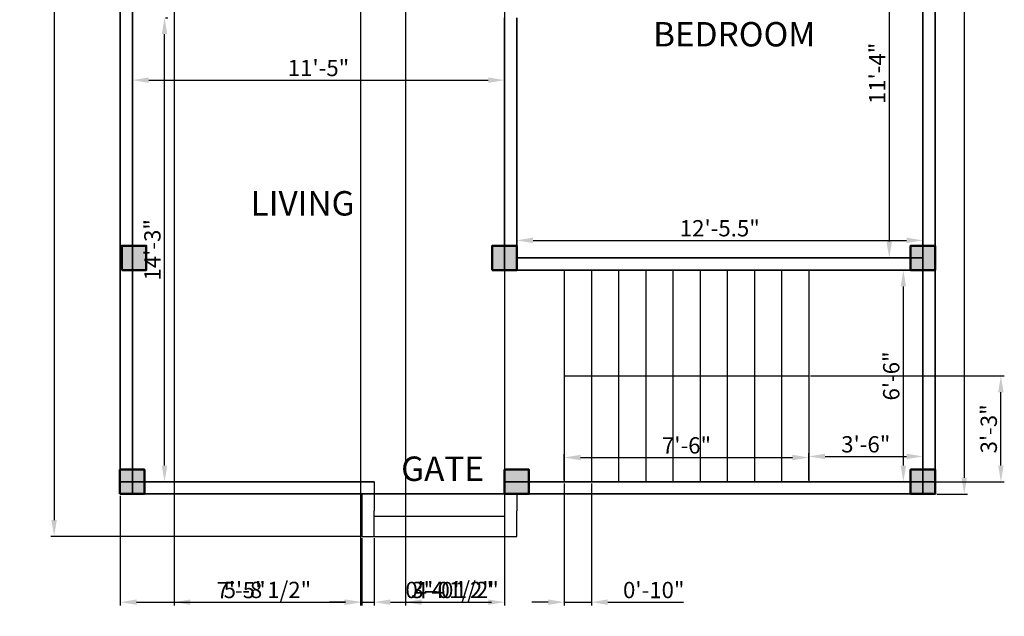
# Model space of a CAD drawing. Units: inches. Extents: x 6892 to 7255, y 6029 to 6556.
# Tile 1 of 2: x 6892 to 7255, y 6029 to 6249. Entities that reach past the tile are written whole.
import ezdxf

# ---------------------------------------------------------------- set-up
doc = ezdxf.new("R2010")
doc.units = ezdxf.units.IN
for name, color, linetype, lineweight in [('A-ANNO-DIMS', 2, 'Continuous', 18), ('A-ANNO-TEXT', 7, 'Continuous', 18), ('A-AREA-IDEN', 7, 'Continuous', 25), ('A-COLS', 7, 'Continuous', 50), ('A-COLS-PATT', 1, 'Continuous', 13), ('A-FLOR-STRS', 7, 'Continuous', 25), ('A-WALL', 7, 'Continuous', 35)]:
    doc.layers.add(name, color=color, linetype=linetype, lineweight=lineweight)
doc.styles.get("Standard").update_dxf_attribs({"font": 'arial.ttf'})
doc.dimstyles.new('ISO-25', dxfattribs={"dimtxt": 6, "dimasz": 6, "dimexe": 1.25, "dimexo": 0.625, "dimtad": 1, "dimlunit": 3, "dimtxsty": 'Standard', "dimcen": 2.5, "dimadec": 0, "dimazin": 0, "dimtfac": 1, "dimtmove": 0, "dimatfit": 3, "dimfxl": 1, "dimarcsym": 0})

# ---------------------------------------------------------------- blocks, each defined once
blk = doc.blocks.new('*D1')
at = {"layer": 'A-ANNO-DIMS', "color": 0, "lineweight": -2, "transparency": 16777216}
for p, q in [((6945.77, 6249.77), (6946.64, 6249.77)), ((6945.39, 6084.77), (6945.39, 6243.77)), ((6945.77, 6078.77), (6946.64, 6078.77))]:
    blk.add_line(p, q, dxfattribs=at)
at = {"layer": 'A-ANNO-DIMS', "color": 0, "transparency": 16777216}
for points in [[(6944.39, 6243.77), (6946.39, 6243.77), (6945.39, 6249.77)], [(6944.39, 6084.77), (6946.39, 6084.77), (6945.39, 6078.77)]]:
    blk.add_solid(points, dxfattribs=at)
at = {"layer": 'Defpoints', "color": 0, "transparency": 16777216}
for p in [(6945.15, 6249.77), (6945.39, 6249.77), (6945.15, 6078.77)]:
    blk.add_point(p, dxfattribs=at)
at = {"layer": 'A-ANNO-DIMS', "color": 0, "transparency": 16777216, "insert": (6941.7, 6164.27), "char_height": 6, "attachment_point": 5, "rotation": 90}
blk.add_mtext('14\'-3"', dxfattribs=at)
blk = doc.blocks.new('*D2')
at = {"layer": 'A-ANNO-DIMS', "color": 0, "lineweight": -2, "transparency": 16777216}
for p, q in [((6933.57, 6227.41), (6933.57, 6228.04)), ((6939.57, 6226.79), (7064.57, 6226.79)), ((7070.57, 6227.41), (7070.57, 6228.04))]:
    blk.add_line(p, q, dxfattribs=at)
at = {"layer": 'A-ANNO-DIMS', "color": 0, "transparency": 16777216}
for points in [[(6939.57, 6227.79), (6939.57, 6225.79), (6933.57, 6226.79)], [(7064.57, 6227.79), (7064.57, 6225.79), (7070.57, 6226.79)]]:
    blk.add_solid(points, dxfattribs=at)
at = {"layer": 'Defpoints', "color": 0, "transparency": 16777216}
for p in [(6933.57, 6226.79), (7070.57, 6226.79), (7070.57, 6226.79)]:
    blk.add_point(p, dxfattribs=at)
at = {"layer": 'A-ANNO-DIMS', "color": 0, "transparency": 16777216, "insert": (7002.07, 6230.48), "char_height": 6, "attachment_point": 5}
blk.add_mtext('11\'-5"', dxfattribs=at)
blk = doc.blocks.new('*D10')
at = {"layer": 'A-ANNO-DIMS', "color": 0, "lineweight": -2, "transparency": 16777216}
for p, q in [((7075.07, 6161.9), (7075.07, 6168.99)), ((7081.07, 6167.74), (7218.57, 6167.74)), ((7224.57, 6161.9), (7224.57, 6168.99))]:
    blk.add_line(p, q, dxfattribs=at)
at = {"layer": 'A-ANNO-DIMS', "color": 0, "transparency": 16777216}
for points in [[(7081.07, 6168.74), (7081.07, 6166.74), (7075.07, 6167.74)], [(7218.57, 6168.74), (7218.57, 6166.74), (7224.57, 6167.74)]]:
    blk.add_solid(points, dxfattribs=at)
at = {"layer": 'Defpoints', "color": 0, "transparency": 16777216}
for p in [(7224.57, 6167.74), (7075.07, 6161.27), (7224.57, 6161.27)]:
    blk.add_point(p, dxfattribs=at)
at = {"layer": 'A-ANNO-DIMS', "color": 0, "transparency": 16777216, "insert": (7149.82, 6171.43), "char_height": 6, "attachment_point": 5}
blk.add_mtext('12\'-5.5"', dxfattribs=at)
blk = doc.blocks.new('*D11')
at = {"layer": 'A-ANNO-DIMS', "color": 0, "lineweight": -2, "transparency": 16777216}
for p, q in [((7223.95, 6297.27), (7210.95, 6297.27)), ((7212.2, 6291.27), (7212.2, 6167.27)), ((7223.95, 6161.27), (7210.95, 6161.27))]:
    blk.add_line(p, q, dxfattribs=at)
at = {"layer": 'A-ANNO-DIMS', "color": 0, "transparency": 16777216}
for points in [[(7211.2, 6291.27), (7213.2, 6291.27), (7212.2, 6297.27)], [(7211.2, 6167.27), (7213.2, 6167.27), (7212.2, 6161.27)]]:
    blk.add_solid(points, dxfattribs=at)
at = {"layer": 'Defpoints', "color": 0, "transparency": 16777216}
for p in [(7224.57, 6297.27), (7212.2, 6161.27), (7224.57, 6161.27)]:
    blk.add_point(p, dxfattribs=at)
at = {"layer": 'A-ANNO-DIMS', "color": 0, "transparency": 16777216, "insert": (7208.56, 6229.27), "char_height": 6, "attachment_point": 5, "rotation": 90}
blk.add_mtext('11\'-4"', dxfattribs=at)
blk = doc.blocks.new('*D12')
at = {"layer": 'A-ANNO-DIMS', "color": 0, "lineweight": -2, "transparency": 16777216}
for p, q in [((7092.57, 6079.4), (7092.57, 6088.96)), ((7098.57, 6087.71), (7176.57, 6087.71)), ((7182.57, 6079.4), (7182.57, 6088.96))]:
    blk.add_line(p, q, dxfattribs=at)
at = {"layer": 'A-ANNO-DIMS', "color": 0, "transparency": 16777216}
for points in [[(7098.57, 6088.71), (7098.57, 6086.71), (7092.57, 6087.71)], [(7176.57, 6088.71), (7176.57, 6086.71), (7182.57, 6087.71)]]:
    blk.add_solid(points, dxfattribs=at)
at = {"layer": 'Defpoints', "color": 0, "transparency": 16777216}
for p in [(7182.57, 6087.71), (7092.57, 6078.77), (7182.57, 6078.77)]:
    blk.add_point(p, dxfattribs=at)
at = {"layer": 'A-ANNO-DIMS', "color": 0, "transparency": 16777216, "insert": (7137.57, 6091.4), "char_height": 6, "attachment_point": 5}
blk.add_mtext('7\'-6"', dxfattribs=at)
blk = doc.blocks.new('*D13')
at = {"layer": 'A-ANNO-DIMS', "color": 0, "lineweight": -2, "transparency": 16777216}
for p, q in [((7182.57, 6079.4), (7182.57, 6089.37)), ((7188.57, 6088.12), (7218.57, 6088.12)), ((7224.57, 6079.4), (7224.57, 6089.37))]:
    blk.add_line(p, q, dxfattribs=at)
at = {"layer": 'A-ANNO-DIMS', "color": 0, "transparency": 16777216}
for points in [[(7188.57, 6089.12), (7188.57, 6087.12), (7182.57, 6088.12)], [(7218.57, 6089.12), (7218.57, 6087.12), (7224.57, 6088.12)]]:
    blk.add_solid(points, dxfattribs=at)
at = {"layer": 'Defpoints', "color": 0, "transparency": 16777216}
for p in [(7224.57, 6088.12), (7182.57, 6078.77), (7224.57, 6078.77)]:
    blk.add_point(p, dxfattribs=at)
at = {"layer": 'A-ANNO-DIMS', "color": 0, "transparency": 16777216, "insert": (7203.57, 6091.81), "char_height": 6, "attachment_point": 5}
blk.add_mtext('3\'-6"', dxfattribs=at)
blk = doc.blocks.new('*D14')
at = {"layer": 'A-ANNO-DIMS', "color": 0, "lineweight": -2, "transparency": 16777216}
for p, q in [((7223.95, 6156.77), (7216.16, 6156.77)), ((7217.41, 6084.77), (7217.41, 6150.77)), ((7223.95, 6078.77), (7216.16, 6078.77))]:
    blk.add_line(p, q, dxfattribs=at)
at = {"layer": 'A-ANNO-DIMS', "color": 0, "transparency": 16777216}
for points in [[(7216.41, 6150.77), (7218.41, 6150.77), (7217.41, 6156.77)], [(7216.41, 6084.77), (7218.41, 6084.77), (7217.41, 6078.77)]]:
    blk.add_solid(points, dxfattribs=at)
at = {"layer": 'Defpoints', "color": 0, "transparency": 16777216}
for p in [(7217.41, 6156.77), (7224.57, 6156.77), (7224.57, 6078.77)]:
    blk.add_point(p, dxfattribs=at)
at = {"layer": 'A-ANNO-DIMS', "color": 0, "transparency": 16777216, "insert": (7213.72, 6117.77), "char_height": 6, "attachment_point": 5, "rotation": 90}
blk.add_mtext('6\'-6"', dxfattribs=at)
blk = doc.blocks.new('*D16')
at = {"layer": 'A-ANNO-DIMS', "color": 0, "lineweight": -2, "transparency": 16777216}
for p, q in [((7229.7, 6506.27), (7241.06, 6506.27)), ((7239.81, 6500.27), (7239.81, 6080.27)), ((7229.7, 6074.27), (7241.06, 6074.27))]:
    blk.add_line(p, q, dxfattribs=at)
at = {"layer": 'A-ANNO-DIMS', "color": 0, "transparency": 16777216}
for points in [[(7238.81, 6500.27), (7240.81, 6500.27), (7239.81, 6506.27)], [(7238.81, 6080.27), (7240.81, 6080.27), (7239.81, 6074.27)]]:
    blk.add_solid(points, dxfattribs=at)
at = {"layer": 'Defpoints', "color": 0, "transparency": 16777216}
for p in [(7229.07, 6506.27), (7229.07, 6074.27), (7239.81, 6074.27)]:
    blk.add_point(p, dxfattribs=at)
at = {"layer": 'A-ANNO-DIMS', "color": 0, "transparency": 16777216, "insert": (7236.12, 6290.27), "char_height": 6, "attachment_point": 5, "rotation": 90}
blk.add_mtext("36'", dxfattribs=at)
blk = doc.blocks.new('COL-9IN-SQ')
blk.add_lwpolyline([(0, 0), (9, 0), (9, 9), (0, 9)], close=True)
blk = doc.blocks.new('*D20')
at = {"layer": 'A-ANNO-DIMS', "color": 0, "lineweight": -2, "transparency": 16777216}
for p, q in [((6928.45, 6506.27), (6903.48, 6506.27)), ((6904.73, 6500.27), (6904.73, 6064.66)), ((7017.45, 6058.66), (6903.48, 6058.66))]:
    blk.add_line(p, q, dxfattribs=at)
at = {"layer": 'A-ANNO-DIMS', "color": 0, "transparency": 16777216}
for points in [[(6903.73, 6500.27), (6905.73, 6500.27), (6904.73, 6506.27)], [(6903.73, 6064.66), (6905.73, 6064.66), (6904.73, 6058.66)]]:
    blk.add_solid(points, dxfattribs=at)
at = {"layer": 'Defpoints', "color": 0, "transparency": 16777216}
for p in [(6929.07, 6506.27), (6904.73, 6058.66), (7018.07, 6058.66)]:
    blk.add_point(p, dxfattribs=at)
at = {"layer": 'A-ANNO-DIMS', "color": 0, "transparency": 16777216, "insert": (6901, 6282.47), "char_height": 6, "attachment_point": 5, "rotation": 90}
blk.add_mtext('37\'-3 1/2"', dxfattribs=at)
blk = doc.blocks.new('*D21')
at = {"layer": 'A-ANNO-DIMS', "color": 0, "lineweight": -2, "transparency": 16777216}
for p, q in [((7022.57, 6058.04), (7022.57, 6033.16)), ((7070.57, 6058.04), (7070.57, 6033.16)), ((7028.57, 6034.41), (7064.57, 6034.41))]:
    blk.add_line(p, q, dxfattribs=at)
at = {"layer": 'A-ANNO-DIMS', "color": 0, "transparency": 16777216}
for points in [[(7028.57, 6035.41), (7028.57, 6033.41), (7022.57, 6034.41)], [(7064.57, 6035.41), (7064.57, 6033.41), (7070.57, 6034.41)]]:
    blk.add_solid(points, dxfattribs=at)
at = {"layer": 'Defpoints', "color": 0, "transparency": 16777216}
for p in [(7022.57, 6058.66), (7070.57, 6058.66), (7070.57, 6034.41)]:
    blk.add_point(p, dxfattribs=at)
at = {"layer": 'A-ANNO-DIMS', "color": 0, "transparency": 16777216, "insert": (7046.57, 6038.1), "char_height": 6, "attachment_point": 5}
blk.add_mtext('4\'-0"', dxfattribs=at)
blk = doc.blocks.new('*D22')
at = {"layer": 'A-ANNO-DIMS', "color": 0, "lineweight": -2, "transparency": 16777216}
for p, q in [((7034.07, 6355.65), (7034.07, 6033.16)), ((7070.6, 6351.27), (7070.6, 6033.16)), ((7040.07, 6034.41), (7064.6, 6034.41))]:
    blk.add_line(p, q, dxfattribs=at)
at = {"layer": 'A-ANNO-DIMS', "color": 0, "transparency": 16777216}
for points in [[(7040.07, 6035.41), (7040.07, 6033.41), (7034.07, 6034.41)], [(7064.6, 6035.41), (7064.6, 6033.41), (7070.6, 6034.41)]]:
    blk.add_solid(points, dxfattribs=at)
at = {"layer": 'Defpoints', "color": 0, "transparency": 16777216}
for p in [(7034.07, 6356.27), (7070.6, 6351.9), (7070.6, 6034.41)]:
    blk.add_point(p, dxfattribs=at)
at = {"layer": 'A-ANNO-DIMS', "color": 0, "transparency": 16777216, "insert": (7052.34, 6038.14), "char_height": 6, "attachment_point": 5}
blk.add_mtext('3\'-0 1/2"', dxfattribs=at)
blk = doc.blocks.new('*D27')
at = {"layer": 'A-ANNO-DIMS', "color": 0, "lineweight": -2, "transparency": 16777216}
for p, q in [((7018.07, 6058.04), (7018.07, 6033.16)), ((7022.57, 6058.04), (7022.57, 6033.16)), ((7012.07, 6034.41), (7006.07, 6034.41)), ((7018.07, 6034.41), (7022.57, 6034.41)), ((7028.57, 6034.41), (7065.75, 6034.41))]:
    blk.add_line(p, q, dxfattribs=at)
at = {"layer": 'A-ANNO-DIMS', "color": 0, "transparency": 16777216}
for points in [[(7012.07, 6035.41), (7012.07, 6033.41), (7018.07, 6034.41)], [(7028.57, 6035.41), (7028.57, 6033.41), (7022.57, 6034.41)]]:
    blk.add_solid(points, dxfattribs=at)
at = {"layer": 'Defpoints', "color": 0, "transparency": 16777216}
for p in [(7018.07, 6058.66), (7022.57, 6058.66), (7022.57, 6034.41)]:
    blk.add_point(p, dxfattribs=at)
at = {"layer": 'A-ANNO-DIMS', "color": 0, "transparency": 16777216, "insert": (7050.16, 6038.14), "char_height": 6, "attachment_point": 5}
blk.add_mtext('0\'-4 1/2"', dxfattribs=at)
blk = doc.blocks.new('*D28')
at = {"layer": 'A-ANNO-DIMS', "color": 0, "lineweight": -2, "transparency": 16777216}
for p, q in [((6948.94, 6335.71), (6948.94, 6033.16)), ((7017.57, 6335.71), (7017.57, 6033.16)), ((6954.94, 6034.41), (7011.57, 6034.41))]:
    blk.add_line(p, q, dxfattribs=at)
at = {"layer": 'A-ANNO-DIMS', "color": 0, "transparency": 16777216}
for points in [[(6954.94, 6035.41), (6954.94, 6033.41), (6948.94, 6034.41)], [(7011.57, 6035.41), (7011.57, 6033.41), (7017.57, 6034.41)]]:
    blk.add_solid(points, dxfattribs=at)
at = {"layer": 'Defpoints', "color": 0, "transparency": 16777216}
for p in [(6948.94, 6336.33), (7017.57, 6336.33), (7017.57, 6034.41)]:
    blk.add_point(p, dxfattribs=at)
at = {"layer": 'A-ANNO-DIMS', "color": 0, "transparency": 16777216, "insert": (6983.26, 6038.14), "char_height": 6, "attachment_point": 5}
blk.add_mtext('5\'-8 1/2"', dxfattribs=at)
blk = doc.blocks.new('*D30')
at = {"layer": 'A-ANNO-DIMS', "color": 0, "lineweight": -2, "transparency": 16777216}
for p, q in [((7092.57, 6078.15), (7092.57, 6033.16)), ((7102.57, 6078.15), (7102.57, 6033.16)), ((7086.57, 6034.41), (7080.57, 6034.41)), ((7092.57, 6034.41), (7102.57, 6034.41)), ((7108.57, 6034.41), (7136.43, 6034.41))]:
    blk.add_line(p, q, dxfattribs=at)
at = {"layer": 'A-ANNO-DIMS', "color": 0, "transparency": 16777216}
for points in [[(7086.57, 6035.41), (7086.57, 6033.41), (7092.57, 6034.41)], [(7108.57, 6035.41), (7108.57, 6033.41), (7102.57, 6034.41)]]:
    blk.add_solid(points, dxfattribs=at)
at = {"layer": 'Defpoints', "color": 0, "transparency": 16777216}
for p in [(7092.57, 6078.77), (7102.57, 6078.77), (7102.57, 6034.41)]:
    blk.add_point(p, dxfattribs=at)
at = {"layer": 'A-ANNO-DIMS', "color": 0, "transparency": 16777216, "insert": (7125.5, 6038.1), "char_height": 6, "attachment_point": 5}
blk.add_mtext('0\'-10"', dxfattribs=at)
blk = doc.blocks.new('*D31')
at = {"layer": 'A-ANNO-DIMS', "color": 0, "lineweight": -2, "transparency": 16777216}
for p, q in [((7183.2, 6117.77), (7254.57, 6117.77)), ((7253.32, 6084.77), (7253.32, 6111.77)), ((7183.2, 6078.77), (7254.57, 6078.77))]:
    blk.add_line(p, q, dxfattribs=at)
at = {"layer": 'A-ANNO-DIMS', "color": 0, "transparency": 16777216}
for points in [[(7252.32, 6111.77), (7254.32, 6111.77), (7253.32, 6117.77)], [(7252.32, 6084.77), (7254.32, 6084.77), (7253.32, 6078.77)]]:
    blk.add_solid(points, dxfattribs=at)
at = {"layer": 'Defpoints', "color": 0, "transparency": 16777216}
for p in [(7182.57, 6117.77), (7253.32, 6117.77), (7182.57, 6078.77)]:
    blk.add_point(p, dxfattribs=at)
at = {"layer": 'A-ANNO-DIMS', "color": 0, "transparency": 16777216, "insert": (7249.63, 6098.27), "char_height": 6, "attachment_point": 5, "rotation": 90}
blk.add_mtext('3\'-3"', dxfattribs=at)
blk = doc.blocks.new('*D32')
at = {"layer": 'A-ANNO-DIMS', "color": 0, "lineweight": -2, "transparency": 16777216}
for p, q in [((6929.07, 6073.65), (6929.07, 6033.16)), ((7018.07, 6058.04), (7018.07, 6033.16)), ((6935.07, 6034.41), (7012.07, 6034.41))]:
    blk.add_line(p, q, dxfattribs=at)
at = {"layer": 'A-ANNO-DIMS', "color": 0, "transparency": 16777216}
for points in [[(6935.07, 6035.41), (6935.07, 6033.41), (6929.07, 6034.41)], [(7012.07, 6035.41), (7012.07, 6033.41), (7018.07, 6034.41)]]:
    blk.add_solid(points, dxfattribs=at)
at = {"layer": 'Defpoints', "color": 0, "transparency": 16777216}
for p in [(6929.07, 6074.27), (7018.07, 6058.66), (7018.07, 6034.41)]:
    blk.add_point(p, dxfattribs=at)
at = {"layer": 'A-ANNO-DIMS', "color": 0, "transparency": 16777216, "insert": (6973.57, 6038.09), "char_height": 6, "attachment_point": 5}
blk.add_mtext('7\'-5"', dxfattribs=at)

msp = doc.modelspace()

# ---------------------------------------------------------------- hatches: boundary and pattern name
at = {"layer": 'A-COLS-PATT'}
h = msp.add_hatch(color=256, dxfattribs=at)
h.dxf.hatch_style = 1
h.paths.add_polyline_path([(7070.574, 6165.771), (7066.074, 6165.771), (7066.074, 6156.771), (7070.574, 6156.771)])
h.paths.add_polyline_path([(7075.074, 6165.771), (7070.574, 6165.771), (7070.574, 6156.771), (7075.074, 6156.771)])
h.paths.add_polyline_path([(6933.574, 6165.771), (6929.638, 6165.771), (6929.638, 6156.771), (6933.574, 6156.771)])
h.paths.add_polyline_path([(6938.638, 6165.771), (6933.574, 6165.771), (6933.574, 6156.771), (6938.638, 6156.771)])
h.paths.add_polyline_path([(7224.574, 6161.271), (7220.074, 6161.271), (7220.074, 6156.771), (7224.574, 6156.771)])
h.paths.add_polyline_path([(7224.574, 6165.771), (7220.074, 6165.771), (7220.074, 6161.271), (7224.574, 6161.271)])
h.paths.add_polyline_path([(7229.074, 6165.771), (7224.574, 6165.771), (7224.574, 6156.771), (7229.074, 6156.771)])
h.paths.add_polyline_path([(7224.574, 6083.271), (7220.074, 6083.271), (7220.074, 6078.771), (7224.574, 6078.771)])
h.paths.add_polyline_path([(7229.074, 6083.271), (7224.574, 6083.271), (7224.574, 6078.771), (7229.074, 6078.771)])
h.paths.add_polyline_path([(7229.074, 6078.771), (7224.574, 6078.771), (7224.574, 6074.271), (7229.074, 6074.271)])
h.paths.add_polyline_path([(7224.574, 6078.771), (7220.074, 6078.771), (7220.074, 6074.271), (7224.574, 6074.271)])
h.paths.add_polyline_path([(6937.983, 6078.771), (6933.574, 6078.771), (6933.574, 6074.271), (6937.983, 6074.271)])
h.paths.add_polyline_path([(6937.983, 6083.271), (6933.574, 6083.271), (6933.574, 6078.771), (6937.983, 6078.771)])
h.paths.add_polyline_path([(6933.574, 6083.271), (6929.074, 6083.271), (6929.074, 6078.771), (6933.574, 6078.771)])
h.paths.add_polyline_path([(6933.574, 6078.771), (6929.074, 6078.771), (6929.074, 6074.271), (6933.574, 6074.271)])
h.paths.add_polyline_path([(7079.562, 6083.271), (7070.562, 6083.271), (7070.562, 6078.771), (7079.562, 6078.771)])
h.paths.add_polyline_path([(7079.562, 6078.771), (7070.574, 6078.771), (7070.574, 6074.271), (7079.562, 6074.271)])

# ---------------------------------------------------------------- linework, layer by layer
at = {"layer": 'A-FLOR-STRS'}
for p, q in [((7092.574, 6156.771), (7092.574, 6078.771)), ((7102.574, 6156.771), (7102.574, 6078.771)), ((7112.574, 6156.771), (7112.574, 6078.771)), ((7122.574, 6156.771), (7122.574, 6078.771)), ((7132.574, 6156.771), (7132.574, 6078.771)), ((7142.574, 6156.771), (7142.574, 6078.771)), ((7152.574, 6156.771), (7152.574, 6078.771)), ((7162.574, 6156.771), (7162.574, 6078.771)), ((7172.574, 6156.771), (7172.574, 6078.771)), ((7182.574, 6156.771), (7182.574, 6078.771)), ((7092.574, 6117.771), (7182.574, 6117.771)), ((7022.574, 6078.771), (7022.574, 6068.103)), ((7070.574, 6078.771), (7070.574, 6068.103)), ((7018.074, 6074.271), (7018.074, 6068.103)), ((7075.074, 6074.271), (7075.074, 6068.103)), ((7018.074, 6068.103), (7018.074, 6058.661)), ((7022.574, 6058.661), (7022.574, 6068.103)), ((7022.574, 6066.125), (7070.574, 6066.125)), ((7070.574, 6068.103), (7070.574, 6058.661)), ((7075.074, 6058.661), (7075.074, 6068.103)), ((7018.074, 6058.661), (7022.574, 6058.661)), ((7022.574, 6058.661), (7070.574, 6058.661)), ((7070.574, 6058.661), (7075.074, 6058.661))]:
    msp.add_line(p, q, dxfattribs=at)
at = {"layer": 'A-WALL'}
for p, q in [((6929.074, 6074.271), (6929.074, 6506.271)), ((7229.074, 6506.271), (7229.074, 6074.271)), ((7224.574, 6501.771), (7224.574, 6074.271)), ((6933.574, 6074.271), (6933.574, 6497.271)), ((7070.574, 6249.771), (7070.574, 6156.771)), ((7075.074, 6249.771), (7075.074, 6156.771)), ((7075.074, 6161.271), (7224.574, 6161.271)), ((7070.574, 6156.771), (7224.574, 6156.771)), ((7022.574, 6078.771), (6929.074, 6078.771)), ((7229.074, 6078.771), (7070.574, 6078.771)), ((7229.074, 6074.271), (6929.074, 6074.271))]:
    msp.add_line(p, q, dxfattribs=at)

# ---------------------------------------------------------------- block references
at = {"layer": 'A-COLS'}
for p in [(6929.639, 6156.771), (7066.074, 6156.771), (7220.074, 6156.771), (6928.983, 6074.271), (7070.562, 6074.271), (7220.074, 6074.271)]:
    msp.add_blockref('COL-9IN-SQ', p, dxfattribs=at)

# ---------------------------------------------------------------- texts
at = {"layer": 'A-ANNO-TEXT', "insert": (7032.499, 6088.078), "char_height": 9, "attachment_point": 1}
msp.add_mtext_dynamic_manual_height_columns('GATE', width=38.07447, gutter_width=12.5, heights=[0], dxfattribs=at)
at = {"layer": 'A-AREA-IDEN', "char_height": 9, "attachment_point": 1}
for s, width, insert in [('BEDROOM', 22.27899, (7125.269, 6248.207)), ('LIVING', 51.99421, (6977.087, 6185.891))]:
    msp.add_mtext_dynamic_manual_height_columns(s, width=width, gutter_width=12.5, heights=[0], dxfattribs=dict(at, insert=insert))

# ---------------------------------------------------------------- dimensions: what is measured, and where the dimension line sits
at = {"layer": 'A-ANNO-DIMS'}
for base, p1, p2, override, picture, middle in [((6904.733, 6058.661), (6929.074, 6506.271), (7018.074, 6058.661), {"dimdec": 1, "dimlfac": 1, "dimrnd": 0, "dimzin": 1, "dimdsep": 46, "dimlunit": 4, "dimfrac": 2}, '*D20', (6901.003, 6282.466)), ((7239.813, 6074.271), (7229.074, 6506.271), (7229.074, 6074.271), {"dimclrd": 0, "dimclre": 0, "dimclrt": 0}, '*D16', (7236.122, 6290.271)), ((7212.202, 6161.271), (7224.574, 6297.271), (7224.574, 6161.271), {"dimclrd": 0, "dimclre": 0, "dimclrt": 0}, '*D11', (7208.565, 6229.271)), ((6945.394, 6249.771), (6945.148, 6078.771), (6945.148, 6249.771), {"dimclrd": 0, "dimclre": 0, "dimclrt": 0}, '*D1', (6941.704, 6164.271)), ((7217.407, 6156.771), (7224.574, 6078.771), (7224.574, 6156.771), {"dimclrd": 0, "dimclre": 0, "dimclrt": 0}, '*D14', (7213.718, 6117.771)), ((7253.324, 6117.771), (7182.574, 6078.771), (7182.574, 6117.771), {"dimdec": 1, "dimlfac": 1, "dimrnd": 0, "dimzin": 1, "dimdsep": 46, "dimlunit": 4, "dimfrac": 2}, '*D31', (7249.633, 6098.271))]:
    dim = msp.add_linear_dim(base=base, p1=p1, p2=p2, angle=90, dimstyle='ISO-25', override=override, dxfattribs=at)
    dim.commit()
    dim.dimension.update_dxf_attribs({"geometry": picture, "text_midpoint": middle})
for base, p1, p2, override, picture, middle in [((7070.605, 6034.411), (7034.074, 6356.271), (7070.605, 6351.898), {"dimdec": 1, "dimlfac": 1, "dimrnd": 0, "dimzin": 1, "dimdsep": 46, "dimlunit": 4, "dimfrac": 2}, '*D22', (7052.339, 6038.14)), ((7017.574, 6034.411), (6948.942, 6336.334), (7017.574, 6336.334), {"dimdec": 1, "dimlfac": 1, "dimrnd": 0, "dimzin": 1, "dimdsep": 46, "dimlunit": 4, "dimfrac": 2}, '*D28', (6983.258, 6038.138)), ((7070.574, 6226.788), (6933.574, 6226.788), (7070.574, 6226.788), {"dimclrd": 0, "dimclre": 0, "dimclrt": 0}, '*D2', (7002.074, 6230.477)), ((7224.574, 6167.737), (7075.074, 6161.271), (7224.574, 6161.271), {"dimclrd": 0, "dimclre": 0, "dimclrt": 0}, '*D10', (7149.824, 6171.425)), ((7182.574, 6087.712), (7092.574, 6078.771), (7182.574, 6078.771), {"dimclrd": 0, "dimclre": 0, "dimclrt": 0}, '*D12', (7137.574, 6091.401)), ((7224.574, 6088.121), (7182.574, 6078.771), (7224.574, 6078.771), {"dimclrd": 0, "dimclre": 0, "dimclrt": 0}, '*D13', (7203.574, 6091.812)), ((7102.574, 6034.411), (7092.574, 6078.771), (7102.574, 6078.771), {"dimdec": 1, "dimlfac": 1, "dimrnd": 0, "dimzin": 1, "dimdsep": 46, "dimlunit": 4, "dimfrac": 2}, '*D30', (7125.504, 6038.099)), ((7018.074, 6034.411), (6929.074, 6074.271), (7018.074, 6058.661), {"dimdec": 1, "dimlfac": 1, "dimrnd": 0, "dimzin": 1, "dimdsep": 46, "dimlunit": 4, "dimfrac": 2}, '*D32', (6973.574, 6038.087)), ((7022.574, 6034.411), (7018.074, 6058.661), (7022.574, 6058.661), {"dimdec": 1, "dimlfac": 1, "dimrnd": 0, "dimzin": 1, "dimdsep": 46, "dimlunit": 4, "dimfrac": 2}, '*D27', (7050.164, 6038.138)), ((7070.574, 6034.411), (7022.574, 6058.661), (7070.574, 6058.661), {"dimdec": 1, "dimlfac": 1, "dimrnd": 0, "dimzin": 1, "dimdsep": 46, "dimlunit": 4, "dimfrac": 2}, '*D21', (7046.574, 6038.099))]:
    dim = msp.add_linear_dim(base=base, p1=p1, p2=p2, dimstyle='ISO-25', override=override, dxfattribs=at)
    dim.commit()
    dim.dimension.update_dxf_attribs({"geometry": picture, "text_midpoint": middle})

doc.saveas('drawing.dxf')
